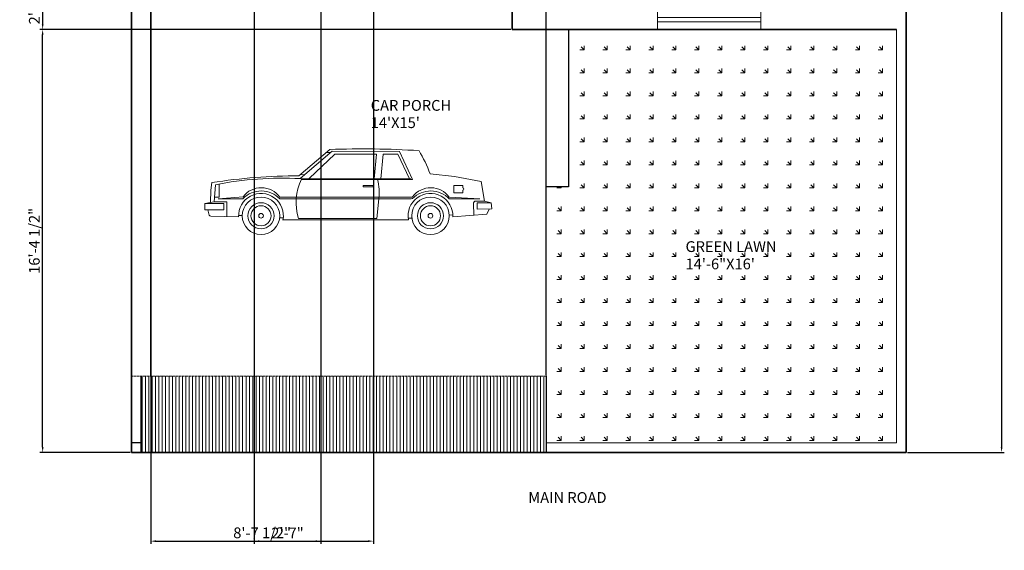
# Model space of a CAD drawing. Units: inches. Extents: x 1265 to 2734, y 1741 to 2595.
# Tile 1 of 10: x 2277 to 2734, y 1741 to 1988. Entities that reach past the tile are written whole.
import ezdxf

# ---------------------------------------------------------------- set-up
doc = ezdxf.new("R2010")
doc.units = ezdxf.units.IN
doc.header["$LTSCALE"] = 0.1
doc.linetypes.add('ACAD_ISO02W100', pattern=[15, 12, -3])
for name, color, linetype, lineweight in [('A-ANNO-DIMS', 2, 'Continuous', 18), ('A-ANNO-TEXT', 7, 'Continuous', 18), ('A-AREA-IDEN', 7, 'Continuous', 18), ('A-GLAZ', 4, 'Continuous', 18), ('A-WALL', 7, 'Continuous', 35), ('C-PROP', 7, 'Continuous', 35), ('C-VEHI', 8, 'Continuous', 15), ('L-HRDS', 8, 'Continuous', 25), ('L-HRDS-OVHD', 8, 'ACAD_ISO02W100', 18), ('L-HRDS-PATT', 252, 'Continuous', 13), ('L-PLNT', 3, 'Continuous', 18), ('L-PLNT-PATT', 94, 'Continuous', 13)]:
    doc.layers.add(name, color=color, linetype=linetype, lineweight=lineweight)
doc.styles.get("Standard").update_dxf_attribs({"font": 'arial.ttf', "height": 5})
doc.dimstyles.new('ISO-25', dxfattribs={"dimtxt": 5, "dimasz": 2.5, "dimexe": 1.25, "dimexo": 0.625, "dimtad": 1, "dimlunit": 3, "dimtxsty": 'Standard', "dimcen": 2.5, "dimadec": 0, "dimazin": 0, "dimtfac": 1, "dimtmove": 0, "dimatfit": 3, "dimfxl": 1, "dimarcsym": 0})

# ---------------------------------------------------------------- blocks, each defined once
blk = doc.blocks.new('*D3')
at = {"layer": 'A-ANNO-DIMS', "color": 0, "lineweight": -2, "transparency": 16777216}
for p, q in [((2689.23, 2542.66), (2734.23, 2542.66)), ((2732.98, 2540.16), (2732.98, 1789.16)), ((2689.23, 1786.66), (2734.23, 1786.66))]:
    blk.add_line(p, q, dxfattribs=at)
at = {"layer": 'A-ANNO-DIMS', "color": 0, "lineweight": 100, "transparency": 16777216}
for points in [[(2732.56, 2540.16), (2733.39, 2540.16), (2732.98, 2542.66)], [(2732.56, 1789.16), (2733.39, 1789.16), (2732.98, 1786.66)]]:
    blk.add_solid(points, dxfattribs=at)
at = {"layer": 'Defpoints', "color": 0, "lineweight": 100, "transparency": 16777216}
for p in [(2688.6, 2542.66), (2688.6, 1786.66), (2732.98, 1786.66)]:
    blk.add_point(p, dxfattribs=at)
at = {"layer": 'A-ANNO-DIMS', "color": 0, "transparency": 16777216, "insert": (2729.8, 2164.66), "char_height": 5, "attachment_point": 5, "rotation": 90}
blk.add_mtext("63'", dxfattribs=at)
blk = doc.blocks.new('WINDOW-48IN')
for p, q in [((0, 9), (0, 0)), ((48, 9), (0, 9)), ((48, 5.5), (0, 5.5)), ((48, 9), (48, 0)), ((48, 3.5), (0, 3.5)), ((0, 0), (48, 0))]:
    blk.add_line(p, q)
blk = doc.blocks.new('*D40')
at = {"layer": 'A-ANNO-DIMS', "color": 0, "lineweight": -2, "transparency": 16777216}
for p, q in [((2504.98, 1983.16), (2286.1, 1983.16)), ((2287.35, 1789.16), (2287.35, 1980.66)), ((2327.98, 1786.66), (2286.1, 1786.66))]:
    blk.add_line(p, q, dxfattribs=at)
at = {"layer": 'A-ANNO-DIMS', "color": 0, "lineweight": 100, "transparency": 16777216}
for points in [[(2286.94, 1980.66), (2287.77, 1980.66), (2287.35, 1983.16)], [(2286.94, 1789.16), (2287.77, 1789.16), (2287.35, 1786.66)]]:
    blk.add_solid(points, dxfattribs=at)
at = {"layer": 'Defpoints', "color": 0, "lineweight": 100, "transparency": 16777216}
for p in [(2287.35, 1983.16), (2505.6, 1983.16), (2328.6, 1786.66)]:
    blk.add_point(p, dxfattribs=at)
at = {"layer": 'A-ANNO-DIMS', "color": 0, "transparency": 16777216, "insert": (2284.14, 1884.91), "char_height": 5, "attachment_point": 5, "rotation": 90}
blk.add_mtext('16\'-4 1/2"', dxfattribs=at)
blk = doc.blocks.new('*D41')
at = {"layer": 'A-ANNO-DIMS', "color": 0, "lineweight": -2, "transparency": 16777216}
for p, q in [((2336.98, 2014.66), (2286.1, 2014.66)), ((2287.35, 2012.16), (2287.35, 1985.66)), ((2504.98, 1983.16), (2286.1, 1983.16))]:
    blk.add_line(p, q, dxfattribs=at)
at = {"layer": 'A-ANNO-DIMS', "color": 0, "lineweight": 100, "transparency": 16777216}
for points in [[(2286.94, 2012.16), (2287.77, 2012.16), (2287.35, 2014.66)], [(2286.94, 1985.66), (2287.77, 1985.66), (2287.35, 1983.16)]]:
    blk.add_solid(points, dxfattribs=at)
at = {"layer": 'Defpoints', "color": 0, "lineweight": 100, "transparency": 16777216}
for p in [(2337.6, 2014.66), (2287.35, 1983.16), (2505.6, 1983.16)]:
    blk.add_point(p, dxfattribs=at)
at = {"layer": 'A-ANNO-DIMS', "color": 0, "transparency": 16777216, "insert": (2284.14, 1998.91), "char_height": 5, "attachment_point": 5, "rotation": 90}
blk.add_mtext('2\'-7 1/2"', dxfattribs=at)
blk = doc.blocks.new('*D42')
at = {"layer": 'A-ANNO-DIMS', "color": 0, "lineweight": -2, "transparency": 16777216}
for p, q in [((2328.6, 1822.68), (2328.6, 2585.16)), ((2521.32, 1822.68), (2521.32, 2585.16)), ((2331.1, 2583.91), (2518.82, 2583.91))]:
    blk.add_line(p, q, dxfattribs=at)
at = {"layer": 'A-ANNO-DIMS', "color": 0, "lineweight": 100, "transparency": 16777216}
for points in [[(2331.1, 2584.32), (2331.1, 2583.49), (2328.6, 2583.91)], [(2518.82, 2584.32), (2518.82, 2583.49), (2521.32, 2583.91)]]:
    blk.add_solid(points, dxfattribs=at)
at = {"layer": 'Defpoints', "color": 0, "lineweight": 100, "transparency": 16777216}
for p in [(2521.32, 2583.91), (2328.6, 1822.06), (2521.32, 1822.06)]:
    blk.add_point(p, dxfattribs=at)
at = {"layer": 'A-ANNO-DIMS', "color": 0, "transparency": 16777216, "insert": (2424.96, 2587.12), "char_height": 5, "attachment_point": 5}
blk.add_mtext('16\'-0 1/2"', dxfattribs=at)
blk = doc.blocks.new('*D43')
at = {"layer": 'A-ANNO-DIMS', "color": 0, "lineweight": -2, "transparency": 16777216}
for p, q in [((2337.6, 2308.03), (2337.6, 1744.16)), ((2441.1, 2308.03), (2441.1, 1744.16)), ((2340.1, 1745.41), (2438.6, 1745.41))]:
    blk.add_line(p, q, dxfattribs=at)
at = {"layer": 'A-ANNO-DIMS', "color": 0, "lineweight": 100, "transparency": 16777216}
for points in [[(2340.1, 1745.82), (2340.1, 1744.99), (2337.6, 1745.41)], [(2438.6, 1745.82), (2438.6, 1744.99), (2441.1, 1745.41)]]:
    blk.add_solid(points, dxfattribs=at)
at = {"layer": 'Defpoints', "color": 0, "lineweight": 100, "transparency": 16777216}
for p in [(2337.6, 2308.66), (2441.1, 2308.66), (2441.1, 1745.41)]:
    blk.add_point(p, dxfattribs=at)
at = {"layer": 'A-ANNO-DIMS', "color": 0, "transparency": 16777216, "insert": (2389.35, 1748.62), "char_height": 5, "attachment_point": 5}
blk.add_mtext('8\'-7 1/2"', dxfattribs=at)
blk = doc.blocks.new('*D45')
at = {"layer": 'A-ANNO-DIMS', "color": 0, "lineweight": -2, "transparency": 16777216}
for p, q in [((2385.6, 2477.53), (2385.6, 1744.16)), ((2416.67, 2477.91), (2416.67, 1744.16)), ((2388.1, 1745.41), (2414.17, 1745.41))]:
    blk.add_line(p, q, dxfattribs=at)
at = {"layer": 'A-ANNO-DIMS', "color": 0, "lineweight": 100, "transparency": 16777216}
for points in [[(2388.1, 1745.82), (2388.1, 1744.99), (2385.6, 1745.41)], [(2414.17, 1745.82), (2414.17, 1744.99), (2416.67, 1745.41)]]:
    blk.add_solid(points, dxfattribs=at)
at = {"layer": 'Defpoints', "color": 0, "lineweight": 100, "transparency": 16777216}
for p in [(2385.6, 2478.16), (2416.67, 2478.54), (2416.67, 1745.41)]:
    blk.add_point(p, dxfattribs=at)
at = {"layer": 'A-ANNO-DIMS', "color": 0, "transparency": 16777216, "insert": (2401.14, 1748.54), "char_height": 5, "attachment_point": 5}
blk.add_mtext('2\'-7"', dxfattribs=at)
blk = doc.blocks.new('*D48')
at = {"layer": 'A-ANNO-DIMS', "color": 0, "lineweight": -2, "transparency": 16777216}
for p, q in [((2337.6, 2014.03), (2337.6, 1744.16)), ((2441.1, 2014.03), (2441.1, 1744.16)), ((2340.1, 1745.41), (2438.6, 1745.41))]:
    blk.add_line(p, q, dxfattribs=at)
at = {"layer": 'A-ANNO-DIMS', "color": 0, "lineweight": 100, "transparency": 16777216}
for points in [[(2340.1, 1745.82), (2340.1, 1744.99), (2337.6, 1745.41)], [(2438.6, 1745.82), (2438.6, 1744.99), (2441.1, 1745.41)]]:
    blk.add_solid(points, dxfattribs=at)
at = {"layer": 'Defpoints', "color": 0, "lineweight": 100, "transparency": 16777216}
for p in [(2337.6, 2014.66), (2441.1, 2014.66), (2441.1, 1745.41)]:
    blk.add_point(p, dxfattribs=at)
at = {"layer": 'A-ANNO-DIMS', "color": 0, "transparency": 16777216, "insert": (2389.35, 1748.62), "char_height": 5, "attachment_point": 5}
blk.add_mtext('8\'-7 1/2"', dxfattribs=at)

msp = doc.modelspace()

# ---------------------------------------------------------------- hatches: boundary and pattern name
at = {"layer": 'L-HRDS-PATT'}
h = msp.add_hatch(dxfattribs=at)
h.set_pattern_fill('LINE', color=256, scale=0.49, angle=90)
h.paths.add_polyline_path([(2521.319, 1822.059), (2333.102, 1822.059), (2333.102, 1786.657), (2521.319, 1786.657)])
at = {"layer": 'L-PLNT-PATT'}
h = msp.add_hatch(dxfattribs=at)
h.set_pattern_fill('GRASS', color=256, scale=0.42, angle=45)
h.paths.add_polyline_path([(2684.102, 1983.157), (2531.707, 1983.157), (2531.707, 1910.013), (2521.319, 1910.013), (2521.319, 1822.059), (2521.319, 1791.157), (2684.102, 1791.157)])

# ---------------------------------------------------------------- linework, layer by layer
at = {"layer": 'A-WALL'}
for q in [(2505.602, 2014.657), (2684.102, 1983.157)]:
    msp.add_line((2505.602, 1983.157), q, dxfattribs=at)
at = {"layer": 'C-PROP'}
for p, q in [((2328.602, 1786.657), (2328.602, 2542.657)), ((2688.602, 2542.657), (2688.602, 1786.657)), ((2688.602, 1786.657), (2328.602, 1786.657))]:
    msp.add_line(p, q, dxfattribs=at)
at = {"layer": 'C-VEHI'}
for p, q in [((2420.773, 1927.358), (2406.393, 1915.049)), ((2421.952, 1926.54), (2407.016, 1913.82)), ((2421.952, 1926.54), (2453.122, 1926.394)), ((2453.122, 1926.394), (2459.15, 1913.435)), ((2423.108, 1925.213), (2411.279, 1913.915)), ((2421.271, 1925.96), (2419.097, 1925.924)), ((2442.477, 1925.216), (2423.108, 1925.213)), ((2441.474, 1913.791), (2442.477, 1925.216)), ((2444.54, 1913.789), (2445.537, 1925.152)), ((2445.537, 1925.152), (2452.395, 1925.237)), ((2452.395, 1925.237), (2457.818, 1913.778)), ((2458.489, 1913.777), (2407.016, 1913.82)), ((2409.226, 1915.665), (2407.071, 1915.629)), ((2459.15, 1913.435), (2407.782, 1913.435)), ((2478.722, 1914.74), (2467.355, 1916.09)), ((2491.084, 1912.471), (2478.722, 1914.74)), ((2365.449, 1908.46), (2365.362, 1902.704)), ((2365.449, 1908.46), (2366.011, 1911.987)), ((2367.636, 1911.006), (2367.038, 1902.988)), ((2369.354, 1911.333), (2369.354, 1905.208)), ((2440.87, 1910.658), (2436.243, 1910.658)), ((2436.243, 1910.658), (2436.243, 1910.08)), ((2436.243, 1910.08), (2440.87, 1910.08)), ((2440.87, 1910.08), (2440.87, 1910.658)), ((2478.471, 1910.658), (2478.471, 1907.188)), ((2482.636, 1910.658), (2478.471, 1910.658)), ((2482.636, 1909.502), (2482.636, 1910.658)), ((2482.636, 1907.188), (2482.636, 1908.46)), ((2492.675, 1903.386), (2491.084, 1912.471)), ((2369.354, 1905.208), (2367.204, 1905.208)), ((2380.495, 1905.412), (2368.859, 1904.477)), ((2380.495, 1904.477), (2368.859, 1904.477)), ((2397.552, 1905.149), (2458.919, 1905.149)), ((2397.552, 1904.405), (2458.527, 1904.405)), ((2443.647, 1904.411), (2442.722, 1895.271)), ((2458.527, 1904.405), (2459.247, 1904.554)), ((2458.919, 1905.149), (2459.247, 1905.412)), ((2476.304, 1905.221), (2490.45, 1904.405)), ((2476.304, 1904.405), (2490.45, 1904.405)), ((2478.471, 1907.188), (2482.636, 1907.188)), ((2492.675, 1903.386), (2488.692, 1903.386)), ((2495.748, 1902.652), (2492.675, 1903.386)), ((2362.703, 1902.252), (2362.676, 1899.313)), ((2371.538, 1899.313), (2362.676, 1899.313)), ((2367.038, 1902.988), (2362.703, 1902.252)), ((2362.703, 1902.252), (2371.538, 1902.252)), ((2364.064, 1899.364), (2364.72, 1896.88)), ((2367.038, 1902.988), (2372.958, 1903.023)), ((2371.538, 1902.252), (2371.538, 1899.313)), ((2372.958, 1903.023), (2372.957, 1896.15)), ((2487.562, 1902.208), (2487.782, 1896.885)), ((2495.748, 1902.652), (2489.308, 1902.652)), ((2489.308, 1902.652), (2489.308, 1899.659)), ((2489.308, 1899.659), (2496.079, 1899.726)), ((2493.826, 1897.246), (2494.778, 1899.561)), ((2496.079, 1899.726), (2495.748, 1902.652)), ((2365.432, 1896.318), (2378.217, 1896.033)), ((2378.422, 1896.74), (2380.114, 1896.74)), ((2397.457, 1895.597), (2399.267, 1895.597)), ((2399.023, 1894.633), (2457.352, 1894.633)), ((2442.722, 1895.271), (2406.278, 1895.271)), ((2457.238, 1895.393), (2458.926, 1895.388)), ((2476.298, 1896.776), (2477.892, 1897.007)), ((2477.963, 1896.072), (2493.826, 1897.246))]:
    msp.add_line(p, q, dxfattribs=at)
for centre, radius in [((2388.821, 1896.561), 8.727), ((2467.574, 1896.561), 8.727), ((2388.821, 1896.561), 6.072), ((2388.821, 1896.561), 4.659), ((2467.574, 1896.561), 6.072), ((2467.574, 1896.561), 4.659), ((2388.821, 1896.561), 1.084), ((2467.574, 1896.561), 1.084)]:
    msp.add_circle(centre, radius, dxfattribs=at)
for centre, radius, start, end in [((2436.285, 1530.602), 397.059, 86.24967, 92.23894), ((2408.708, 1894.772), 62.401, 19.97614, 30.89345), ((2406.313, 1653.969), 261.146, 89.96542, 98.87787), ((2398.768, 1752.294), 161.736, 87.07682, 101.09777), ((2429.788, 1902.678), 24.649, 153.8259, 197.48762), ((2420.561, 1907.174), 23.251, 353.17556, 15.62185), ((2388.953, 1898.981), 10.625, 35.96693, 142.75278), ((2388.932, 1896.224), 11.856, 43.35672, 135.36298), ((2467.705, 1898.981), 10.625, 35.96693, 142.75278), ((2467.684, 1896.224), 11.856, 43.35672, 135.36298), ((2482.607, 1908.981), 0.521, 273.17983, 86.82017), ((2388.821, 1896.561), 10.401, 348.76626, 182.8486), ((2467.574, 1896.561), 10.401, 357.3058, 190.67853), ((2488.692, 1902.255), 1.131, 90, 182.36883), ((2365.449, 1897.072), 0.754, 194.79404, 268.72236)]:
    msp.add_arc(centre, radius, start, end, dxfattribs=at)
at = {"layer": 'L-HRDS'}
for p, q in [((2337.602, 1822.059), (2337.602, 2014.657)), ((2531.707, 1983.157), (2531.707, 1910.013)), ((2531.707, 1910.013), (2521.454, 1910.013)), ((2333.102, 1786.657), (2333.102, 1822.059)), ((2521.319, 1822.059), (2521.319, 1786.657)), ((2333.102, 1791.157), (2328.602, 1791.157))]:
    msp.add_line(p, q, dxfattribs=at)
at = {"layer": 'L-HRDS-OVHD'}
for p, q in [((2521.319, 1983.157), (2521.319, 1822.059)), ((2521.319, 1822.059), (2328.602, 1822.059))]:
    msp.add_line(p, q, dxfattribs=at)
at = {"layer": 'L-PLNT'}
for p, q in [((2684.102, 1983.157), (2684.102, 1791.157)), ((2684.102, 1791.157), (2521.319, 1791.157))]:
    msp.add_line(p, q, dxfattribs=at)

# ---------------------------------------------------------------- block references
at = {"layer": 'A-GLAZ'}
msp.add_blockref('WINDOW-48IN', (2573.102, 1983.157), dxfattribs=at)

# ---------------------------------------------------------------- texts
at = {"layer": 'A-ANNO-TEXT'}
msp.add_text('MAIN ROAD', height=5, dxfattribs=at).set_placement((2513.022, 1763.193))
at = {"layer": 'A-AREA-IDEN'}
for s, p in [('CAR PORCH', (2439.808, 1945.346)), ("14'X15'", (2439.808, 1937.314)), ('GREEN LAWN', (2586.096, 1879.741)), ('14\'-6"X16\'', (2586.096, 1871.709))]:
    msp.add_text(s, height=5, dxfattribs=at).set_placement(p)

# ---------------------------------------------------------------- dimensions: what is measured, and where the dimension line sits
at = {"layer": 'A-ANNO-DIMS'}
for base, p1, p2, picture, middle in [((2521.319, 2583.907), (2328.602, 1822.059), (2521.319, 1822.059), '*D42', (2424.961, 2587.117)), ((2416.673, 1745.407), (2385.602, 2478.157), (2416.673, 2478.538), '*D45', (2401.138, 1748.542)), ((2441.102, 1745.407), (2337.602, 2308.657), (2441.102, 2308.657), '*D43', (2389.352, 1748.617)), ((2441.102, 1745.407), (2337.602, 2014.657), (2441.102, 2014.657), '*D48', (2389.352, 1748.617))]:
    dim = msp.add_linear_dim(base=base, p1=p1, p2=p2, dimstyle='ISO-25', override={"dimdec": 1, "dimlfac": 1, "dimrnd": 0, "dimzin": 1, "dimdsep": 46, "dimlunit": 4, "dimfrac": 2}, dxfattribs=at)
    dim.commit()
    dim.dimension.update_dxf_attribs({"geometry": picture, "text_midpoint": middle})
for base, p1, p2, override, picture, middle in [((2732.978, 1786.657), (2688.602, 2542.657), (2688.602, 1786.657), {"dimclrd": 0, "dimclre": 0, "dimclrt": 0}, '*D3', (2729.798, 2164.657)), ((2287.352, 1983.157), (2337.602, 2014.657), (2505.602, 1983.157), {"dimdec": 1, "dimlfac": 1, "dimrnd": 0, "dimzin": 1, "dimdsep": 46, "dimlunit": 4, "dimfrac": 2}, '*D41', (2284.142, 1998.907)), ((2287.352, 1983.157), (2328.602, 1786.657), (2505.602, 1983.157), {"dimdec": 1, "dimlfac": 1, "dimrnd": 0, "dimzin": 1, "dimdsep": 46, "dimlunit": 4, "dimfrac": 2}, '*D40', (2284.142, 1884.907))]:
    dim = msp.add_linear_dim(base=base, p1=p1, p2=p2, angle=90, dimstyle='ISO-25', override=override, dxfattribs=at)
    dim.commit()
    dim.dimension.update_dxf_attribs({"geometry": picture, "text_midpoint": middle})

doc.saveas('drawing.dxf')
